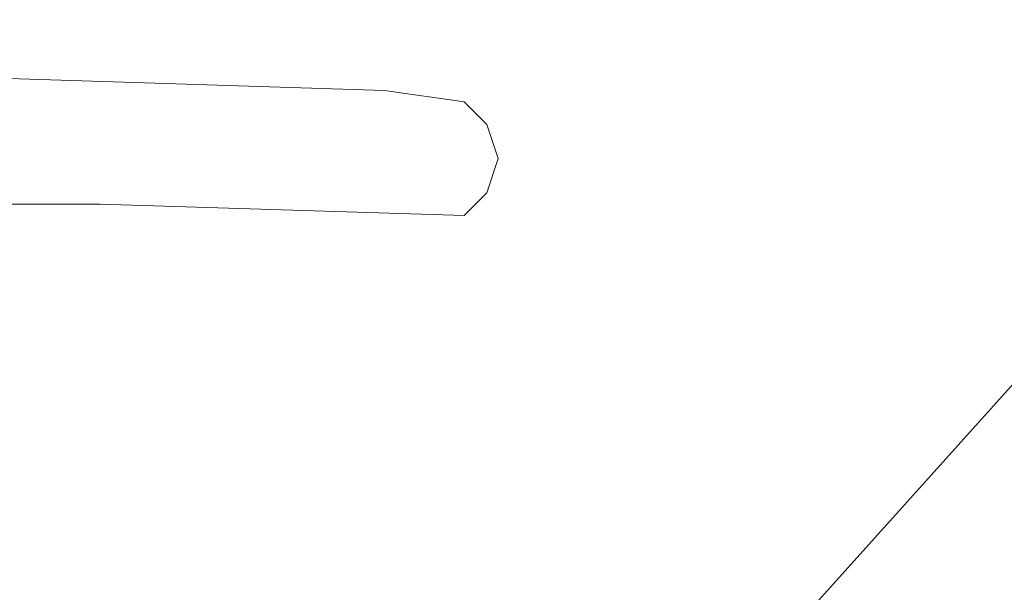
# Model space of a CAD drawing. Units: inches. Extents: x 375 to 1122, y 27 to 1069.
# Tile 117 of 155: x 715.443 to 720.771, y 886.613 to 889.713. Entities that reach past the tile are written whole.
import ezdxf

# ---------------------------------------------------------------- set-up
doc = ezdxf.new("R2010")
doc.units = ezdxf.units.IN
doc.layers.add('Furniture', color=30, linetype='Continuous', lineweight=18)

# ---------------------------------------------------------------- blocks, each defined once
blk = doc.blocks.new('A$C403C54AD')
blk.add_line((0.95931, 1.17062, -0.0006), (1.35847, 0.81256, -0.0006))
blk.add_circle((1.40208, 1.00844, -0.0006), 0.12331)
for points, invisible_edges in [([(1.23412, 0.8271, -0.0249), (1.23412, 0.8271, -0.0249), (1.23874, 0.82556, -0.0249), (1.22951, 0.82556, -0.0249)], 4), ([(1.23412, 0.8271, -0.02644), (1.23412, 0.8271, -0.02644), (1.23874, 0.82556, -0.02644), (1.22951, 0.82556, -0.02644)], 4), ([(1.23412, 0.8271, -0.0249), (1.23412, 0.8271, -0.02644), (1.22951, 0.82556, -0.02644), (1.22951, 0.82556, -0.0249)], 4), ([(1.23874, 0.82556, -0.02644), (1.23874, 0.82556, -0.0249), (1.23412, 0.8271, -0.0249), (1.23412, 0.8271, -0.02644)], 1), ([(1.23874, 0.82556, -0.0249), (1.22951, 0.82556, -0.0249), (1.22643, 0.82248, -0.0249), (1.24182, 0.82248, -0.0249)], 5), ([(1.23874, 0.82556, -0.02644), (1.22951, 0.82556, -0.02644), (1.22643, 0.82248, -0.02644), (1.24182, 0.82248, -0.02644)], 5), ([(1.22951, 0.82556, -0.02644), (1.22951, 0.82556, -0.0249), (1.22643, 0.82248, -0.0249), (1.22643, 0.82248, -0.02644)], 5), ([(1.24182, 0.82248, -0.0249), (1.24182, 0.82248, -0.02644), (1.23874, 0.82556, -0.02644), (1.23874, 0.82556, -0.0249)], 5), ([(1.22643, 0.82248, -0.0249), (1.24182, 0.82248, -0.0249), (1.24028, 0.77323, -0.0249), (1.22489, 0.81171, -0.0249)], 5), ([(1.22643, 0.82248, -0.02644), (1.24182, 0.82248, -0.02644), (1.24028, 0.77323, -0.02644), (1.22489, 0.81171, -0.02644)], 5), ([(1.22643, 0.82248, -0.0249), (1.22643, 0.82248, -0.02644), (1.22489, 0.81171, -0.02644), (1.22489, 0.81171, -0.0249)], 5), ([(1.24028, 0.77323, -0.02644), (1.24028, 0.77323, -0.0249), (1.24182, 0.82248, -0.0249), (1.24182, 0.82248, -0.02644)], 5), ([(1.24028, 0.77323, -0.0249), (1.22489, 0.81171, -0.0249), (1.22181, 0.71474, -0.0249), (1.24028, 0.71474, -0.0249)], 5), ([(1.24028, 0.77323, -0.02644), (1.22489, 0.81171, -0.02644), (1.22181, 0.71474, -0.02644), (1.24028, 0.71474, -0.02644)], 5), ([(1.22489, 0.81171, -0.02644), (1.22489, 0.81171, -0.0249), (1.22181, 0.71474, -0.0249), (1.22181, 0.71474, -0.02644)], 5), ([(1.24028, 0.71474, -0.0249), (1.24028, 0.71474, -0.02644), (1.24028, 0.77323, -0.02644), (1.24028, 0.77323, -0.0249)], 5)]:
    blk.add_3dface(points, dxfattribs=dict(invisible_edges=invisible_edges))

msp = doc.modelspace()

# ---------------------------------------------------------------- block references
at = {"layer": 'Furniture', "xscale": 39.9918517141215, "yscale": 39.9918517141215, "zscale": 39.9918517141215, "rotation": 270}
msp.add_blockref('A$C403C54AD', (684.9549, 938.3156, 0.024), dxfattribs=at)

doc.saveas('drawing.dxf')
